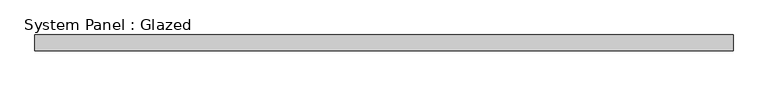
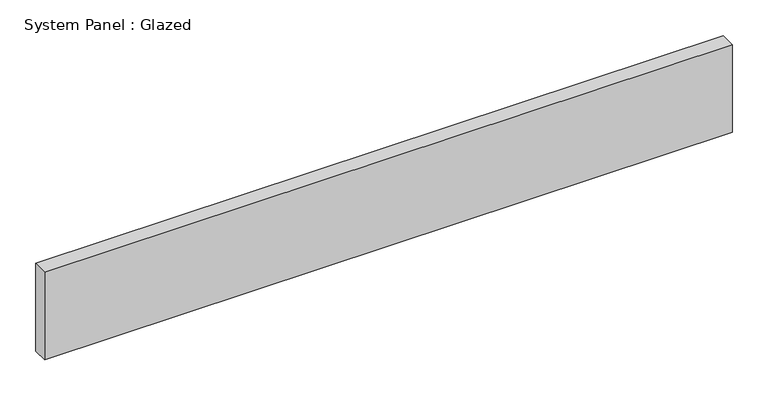
"""IFC4 building model written with IfcOpenShell, lengths in millimetres: plate geometry, System Panel : Glazed."""

from ifc_helpers import new_model, si_unit, origin, origin_with_axes, place, context, project, spatial, polyline, outline, extrude, source, transform, mapped, element, save


def system_panel_glazed_82719d7e(model_context):
    return source(origin(), model_context, "Body", "SweptSolid", [
        extrude(outline(polyline([(556.814808, 24.5), (-556.814808, 24.5), (-556.814808, 49.5), (556.814808, 49.5), (556.814808, 24.5)])), origin_with_axes(), (0.0, 0.0, 1.0), 150.0429688),
    ])


if __name__ == "__main__":
    model = new_model("IFC4")
    model_context = context("Model", 3, world=origin())
    ifc_project = project(units=[si_unit("LENGTHUNIT", "METRE", prefix="MILLI")], contexts=[model_context])
    site = spatial("IfcSite", under=ifc_project)
    building = spatial("IfcBuilding", under=site)
    placement = place(None, origin())
    system_panel_glazed_shape = system_panel_glazed_82719d7e(model_context)
    element("IfcPlate", 1, ObjectType="System Panel : Glazed", at=placement, inside=building, context=model_context, shape_type="MappedRepresentation", body=[
        mapped(system_panel_glazed_shape, transform((0.0, 0.0, 0.0), x_axis=(1.0, 0.0, 0.0), y_axis=(0.0, 1.0, 0.0), z_axis=(0.0, 0.0, 1.0))),
    ])
    save(model, "model.ifc")

# Revit data of these elements
# Type "System Panel : Glazed"
#   Keynote = "H11"
#   Construction Type Id = "GSP4R"
#   Analytic Construction = "1/8 in Pilkington single glazing"
#   Visual Light Transmittance = 0.9
#   Solar Heat Gain Coefficient = 0.86
#   Heat Transfer Coefficient (U) = 6.7069 W/(m²·K)
#   Define Thermal Properties by = 1
# Element 1 (IfcPlate, "System Panel : Glazed")
#   Materials on its faces: "Glass"
# Materials
#   "Glass": class "Glass", colour RGB 0 128 192, transparency 0.9, Description = "Soda Lime Glass", Cost = 0
